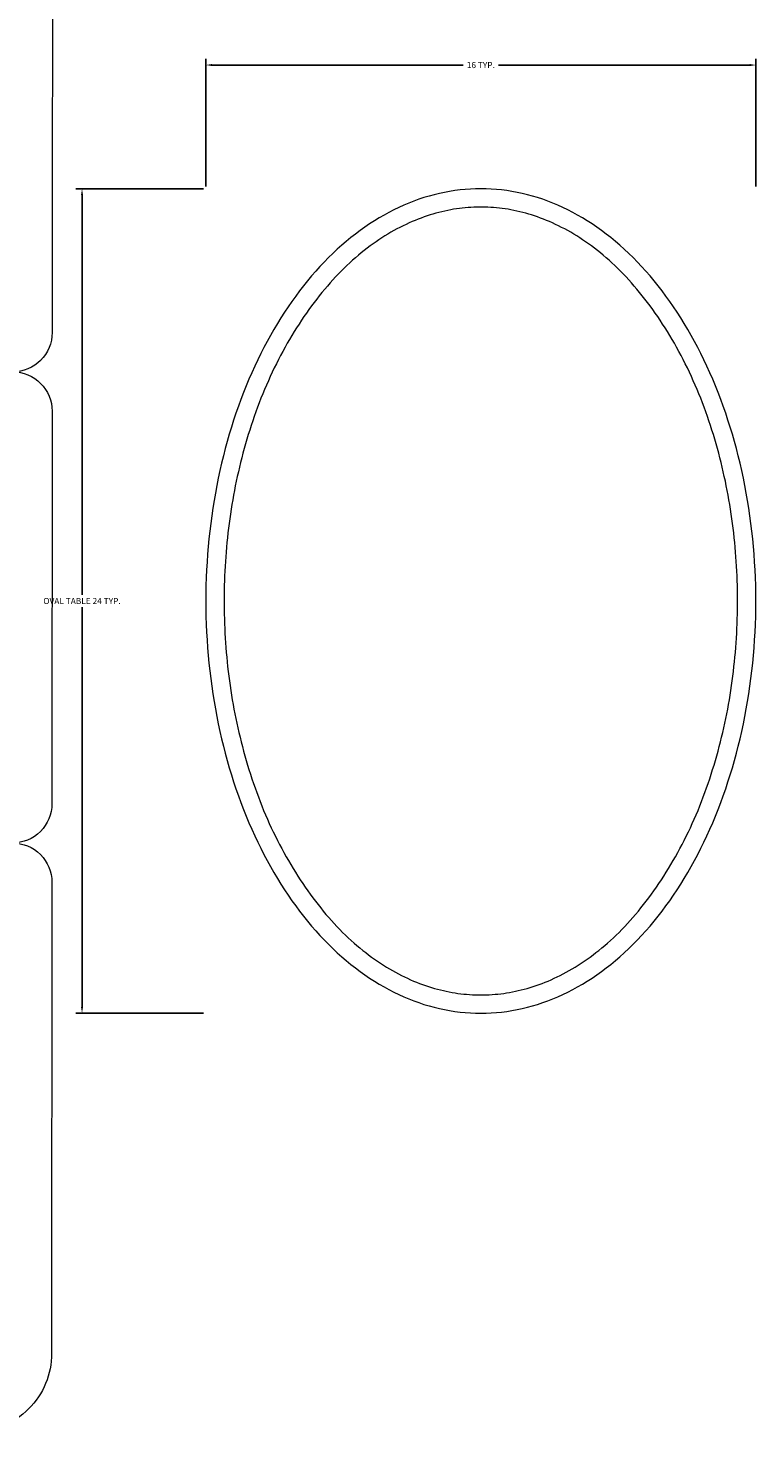
# Model space of a CAD drawing. Units: inches. Extents: x 963 to 2075, y 289 to 2657.
# Tile 84 of 98: x 1533 to 1555, y 2243 to 2284. Entities that reach past the tile are written whole.
import ezdxf

# ---------------------------------------------------------------- set-up
doc = ezdxf.new("R2010")
doc.units = ezdxf.units.IN
doc.layers.add('A-ANNO-DIMS', color=2, linetype='Continuous', lineweight=18)
doc.layers.add('A-FURN', color=8, linetype='Continuous', lineweight=18)
doc.styles.get("Standard").update_dxf_attribs({"font": 'arial.ttf'})
doc.dimstyles.get("Standard").update_dxf_attribs({"dimtxt": 0.18, "dimasz": 0.18, "dimexe": 0.18, "dimexo": 0.0625, "dimgap": 0.09, "dimtad": 0, "dimtih": 1, "dimtoh": 1, "dimdec": 4, "dimzin": 0, "dimdsep": 46, "dimtxsty": 'Standard', "dimcen": 0.09, "dimadec": 0, "dimazin": 0, "dimtfac": 1, "dimtdec": 4, "dimtofl": 0, "dimtmove": 0, "dimatfit": 3, "dimfxl": 1, "dimtolj": 1, "dimtzin": 0, "dimarcsym": 0})

# ---------------------------------------------------------------- blocks, each defined once
blk = doc.blocks.new('SOFA-3SEAT')
at = {"ltscale": 0.03}
blk.add_lwpolyline([(2.442, 16.426, -0.414214), (0.124, 18.743), (0.124, 32.649, -0.414214), (1.283, 33.808, -0.414214), (0.124, 34.967), (0.124, 46.555, -0.414214), (1.283, 47.713, -0.414214), (0.124, 48.872), (0.124, 62.778, -0.414214), (2.442, 65.095), (16.347, 65.095, -0.414214), (18.665, 62.778), (18.665, 18.743, -0.414214), (16.347, 16.426)], format="xyb", close=True, dxfattribs=at)
blk = doc.blocks.new('TABLE-OVAL')
at = {"ltscale": 0.03}
blk.add_polyline3d([(7.656, -0.197, 0), (7.809, -0.194, 0), (7.963, -0.188, 0), (8.116, -0.177, 0), (8.269, -0.162, 0), (8.422, -0.142, 0), (8.575, -0.118, 0), (8.727, -0.09, 0), (8.879, -0.057, 0), (9.031, -0.021, 0), (9.182, 0.021, 0), (9.332, 0.066, 0), (9.482, 0.116, 0), (9.632, 0.17, 0), (9.78, 0.228, 0), (9.928, 0.29, 0), (10.075, 0.357, 0), (10.221, 0.428, 0), (10.366, 0.503, 0), (10.51, 0.582, 0), (10.653, 0.665, 0), (10.796, 0.752, 0), (10.937, 0.843, 0), (11.076, 0.938, 0), (11.215, 1.037, 0), (11.352, 1.14, 0), (11.488, 1.247, 0), (11.623, 1.358, 0), (11.756, 1.472, 0), (11.888, 1.59, 0), (12.018, 1.712, 0), (12.147, 1.838, 0), (12.274, 1.967, 0), (12.399, 2.1, 0), (12.523, 2.237, 0), (12.645, 2.376, 0), (12.765, 2.52, 0), (12.883, 2.666, 0), (13, 2.817, 0), (13.114, 2.97, 0), (13.227, 3.126, 0), (13.337, 3.286, 0), (13.446, 3.449, 0), (13.552, 3.615, 0), (13.657, 3.784, 0), (13.759, 3.955, 0), (13.859, 4.13, 0), (13.957, 4.308, 0), (14.052, 4.488, 0), (14.145, 4.671, 0), (14.236, 4.856, 0), (14.325, 5.044, 0), (14.411, 5.235, 0), (14.495, 5.428, 0), (14.576, 5.623, 0), (14.655, 5.821, 0), (14.731, 6.021, 0), (14.805, 6.222, 0), (14.877, 6.426, 0), (14.945, 6.632, 0), (15.011, 6.84, 0), (15.075, 7.05, 0), (15.135, 7.261, 0), (15.193, 7.475, 0), (15.249, 7.689, 0), (15.301, 7.906, 0), (15.351, 8.123, 0), (15.399, 8.343, 0), (15.443, 8.563, 0), (15.485, 8.785, 0), (15.523, 9.007, 0), (15.559, 9.231, 0), (15.592, 9.456, 0), (15.623, 9.682, 0), (15.65, 9.908, 0), (15.675, 10.136, 0), (15.697, 10.364, 0), (15.715, 10.592, 0), (15.731, 10.821, 0), (15.744, 11.051, 0), (15.755, 11.28, 0), (15.762, 11.51, 0), (15.766, 11.741, 0), (15.768, 11.971, 0), (15.766, 12.201, 0), (15.762, 12.431, 0), (15.755, 12.661, 0), (15.744, 12.891, 0), (15.731, 13.12, 0), (15.715, 13.349, 0), (15.697, 13.578, 0), (15.675, 13.806, 0), (15.65, 14.033, 0), (15.623, 14.26, 0), (15.592, 14.486, 0), (15.559, 14.71, 0), (15.523, 14.934, 0), (15.485, 15.157, 0), (15.443, 15.379, 0), (15.399, 15.599, 0), (15.351, 15.818, 0), (15.301, 16.036, 0), (15.249, 16.252, 0), (15.193, 16.467, 0), (15.135, 16.68, 0), (15.075, 16.892, 0), (15.011, 17.101, 0), (14.945, 17.309, 0), (14.877, 17.515, 0), (14.805, 17.719, 0), (14.731, 17.921, 0), (14.655, 18.121, 0), (14.576, 18.318, 0), (14.495, 18.514, 0), (14.411, 18.707, 0), (14.325, 18.897, 0), (14.236, 19.085, 0), (14.145, 19.271, 0), (14.052, 19.454, 0), (13.957, 19.634, 0), (13.859, 19.811, 0), (13.759, 19.986, 0), (13.657, 20.158, 0), (13.552, 20.327, 0), (13.446, 20.493, 0), (13.337, 20.656, 0), (13.227, 20.815, 0), (13.114, 20.972, 0), (13, 21.125, 0), (12.883, 21.275, 0), (12.765, 21.422, 0), (12.645, 21.565, 0), (12.523, 21.705, 0), (12.399, 21.842, 0), (12.274, 21.974, 0), (12.147, 22.104, 0), (12.018, 22.229, 0), (11.888, 22.351, 0), (11.756, 22.47, 0), (11.623, 22.584, 0), (11.488, 22.695, 0), (11.352, 22.802, 0), (11.215, 22.905, 0), (11.076, 23.004, 0), (10.937, 23.099, 0), (10.796, 23.19, 0), (10.653, 23.277, 0), (10.51, 23.36, 0), (10.366, 23.439, 0), (10.221, 23.514, 0), (10.075, 23.585, 0), (9.928, 23.651, 0), (9.78, 23.714, 0), (9.632, 23.772, 0), (9.482, 23.826, 0), (9.332, 23.876, 0), (9.182, 23.921, 0), (9.031, 23.962, 0), (8.879, 23.999, 0), (8.727, 24.032, 0), (8.575, 24.06, 0), (8.422, 24.084, 0), (8.269, 24.103, 0), (8.116, 24.119, 0), (7.963, 24.13, 0), (7.809, 24.136, 0), (7.656, 24.138, 0), (7.502, 24.136, 0), (7.349, 24.13, 0), (7.196, 24.119, 0), (7.042, 24.103, 0), (6.89, 24.084, 0), (6.737, 24.06, 0), (6.585, 24.032, 0), (6.433, 23.999, 0), (6.281, 23.962, 0), (6.13, 23.921, 0), (5.979, 23.876, 0), (5.83, 23.826, 0), (5.68, 23.772, 0), (5.532, 23.714, 0), (5.384, 23.651, 0), (5.237, 23.585, 0), (5.091, 23.514, 0), (4.946, 23.439, 0), (4.802, 23.36, 0), (4.658, 23.277, 0), (4.516, 23.19, 0), (4.375, 23.099, 0), (4.236, 23.004, 0), (4.097, 22.905, 0), (3.96, 22.802, 0), (3.824, 22.695, 0), (3.689, 22.584, 0), (3.556, 22.47, 0), (3.424, 22.351, 0), (3.294, 22.229, 0), (3.165, 22.104, 0), (3.038, 21.974, 0), (2.913, 21.842, 0), (2.789, 21.705, 0), (2.667, 21.565, 0), (2.547, 21.422, 0), (2.429, 21.275, 0), (2.312, 21.125, 0), (2.198, 20.972, 0), (2.085, 20.815, 0), (1.975, 20.656, 0), (1.866, 20.493, 0), (1.76, 20.327, 0), (1.655, 20.158, 0), (1.553, 19.986, 0), (1.453, 19.811, 0), (1.355, 19.634, 0), (1.26, 19.454, 0), (1.166, 19.271, 0), (1.076, 19.085, 0), (0.987, 18.897, 0), (0.901, 18.707, 0), (0.817, 18.514, 0), (0.736, 18.318, 0), (0.657, 18.121, 0), (0.58, 17.921, 0), (0.507, 17.719, 0), (0.435, 17.515, 0), (0.367, 17.309, 0), (0.301, 17.101, 0), (0.237, 16.892, 0), (0.177, 16.68, 0), (0.118, 16.467, 0), (0.063, 16.252, 0), (0.01, 16.036, 0), (-0.039, 15.818, 0), (-0.087, 15.599, 0), (-0.131, 15.379, 0), (-0.173, 15.157, 0), (-0.211, 14.934, 0), (-0.247, 14.71, 0), (-0.281, 14.486, 0), (-0.311, 14.26, 0), (-0.338, 14.033, 0), (-0.363, 13.806, 0), (-0.385, 13.578, 0), (-0.403, 13.349, 0), (-0.419, 13.12, 0), (-0.432, 12.891, 0), (-0.443, 12.661, 0), (-0.45, 12.431, 0), (-0.454, 12.201, 0), (-0.456, 11.971, 0), (-0.454, 11.741, 0), (-0.45, 11.51, 0), (-0.443, 11.28, 0), (-0.432, 11.051, 0), (-0.419, 10.821, 0), (-0.403, 10.592, 0), (-0.385, 10.364, 0), (-0.363, 10.136, 0), (-0.338, 9.908, 0), (-0.311, 9.682, 0), (-0.281, 9.456, 0), (-0.247, 9.231, 0), (-0.211, 9.007, 0), (-0.173, 8.785, 0), (-0.131, 8.563, 0), (-0.087, 8.343, 0), (-0.039, 8.123, 0), (0.01, 7.906, 0), (0.063, 7.689, 0), (0.118, 7.475, 0), (0.177, 7.261, 0), (0.237, 7.05, 0), (0.301, 6.84, 0), (0.367, 6.632, 0), (0.435, 6.426, 0), (0.507, 6.222, 0), (0.58, 6.021, 0), (0.657, 5.821, 0), (0.736, 5.623, 0), (0.817, 5.428, 0), (0.901, 5.235, 0), (0.987, 5.044, 0), (1.076, 4.856, 0), (1.166, 4.671, 0), (1.26, 4.488, 0), (1.355, 4.308, 0), (1.453, 4.13, 0), (1.553, 3.955, 0), (1.655, 3.784, 0), (1.76, 3.615, 0), (1.866, 3.449, 0), (1.975, 3.286, 0), (2.085, 3.126, 0), (2.198, 2.97, 0), (2.312, 2.817, 0), (2.429, 2.666, 0), (2.547, 2.52, 0), (2.667, 2.376, 0), (2.789, 2.237, 0), (2.913, 2.1, 0), (3.038, 1.967, 0), (3.165, 1.838, 0), (3.294, 1.712, 0), (3.424, 1.59, 0), (3.556, 1.472, 0), (3.689, 1.358, 0), (3.824, 1.247, 0), (3.96, 1.14, 0), (4.097, 1.037, 0), (4.236, 0.938, 0), (4.375, 0.843, 0), (4.516, 0.752, 0), (4.658, 0.665, 0), (4.802, 0.582, 0), (4.946, 0.503, 0), (5.091, 0.428, 0), (5.237, 0.357, 0), (5.384, 0.29, 0), (5.532, 0.228, 0), (5.68, 0.17, 0), (5.83, 0.116, 0), (5.979, 0.066, 0), (6.13, 0.021, 0), (6.281, -0.021, 0), (6.433, -0.057, 0), (6.585, -0.09, 0), (6.737, -0.118, 0), (6.89, -0.142, 0), (7.042, -0.162, 0), (7.196, -0.177, 0), (7.349, -0.188, 0), (7.502, -0.194, 0), (7.656, -0.197, 0)], dxfattribs=at)
blk.add_polyline3d([(7.656, 0.344, 0), (7.739, 0.345, 0), (7.822, 0.347, 0), (7.906, 0.351, 0), (7.99, 0.356, 0), (8.074, 0.362, 0), (8.159, 0.37, 0), (8.244, 0.38, 0), (8.33, 0.391, 0), (8.415, 0.404, 0), (8.501, 0.418, 0), (8.588, 0.434, 0), (8.674, 0.451, 0), (8.761, 0.47, 0), (8.848, 0.491, 0), (8.935, 0.513, 0), (9.023, 0.538, 0), (9.11, 0.563, 0), (9.198, 0.591, 0), (9.286, 0.62, 0), (9.375, 0.651, 0), (9.463, 0.684, 0), (9.552, 0.719, 0), (9.64, 0.755, 0), (9.729, 0.794, 0), (9.818, 0.834, 0), (9.907, 0.876, 0), (9.995, 0.92, 0), (10.084, 0.966, 0), (10.173, 1.013, 0), (10.262, 1.063, 0), (10.35, 1.114, 0), (10.439, 1.167, 0), (10.527, 1.222, 0), (10.615, 1.279, 0), (10.703, 1.338, 0), (10.791, 1.398, 0), (10.878, 1.461, 0), (10.965, 1.525, 0), (11.052, 1.592, 0), (11.139, 1.66, 0), (11.225, 1.73, 0), (11.311, 1.802, 0), (11.396, 1.876, 0), (11.481, 1.952, 0), (11.565, 2.03, 0), (11.649, 2.109, 0), (11.733, 2.191, 0), (11.815, 2.275, 0), (11.898, 2.361, 0), (11.98, 2.448, 0), (12.061, 2.537, 0), (12.141, 2.629, 0), (12.221, 2.721, 0), (12.301, 2.816, 0), (12.379, 2.912, 0), (12.457, 3.01, 0), (12.535, 3.11, 0), (12.611, 3.211, 0), (12.687, 3.314, 0), (12.762, 3.418, 0), (12.836, 3.524, 0), (12.909, 3.632, 0), (12.982, 3.741, 0), (13.053, 3.851, 0), (13.124, 3.963, 0), (13.194, 4.076, 0), (13.262, 4.191, 0), (13.33, 4.307, 0), (13.397, 4.424, 0), (13.463, 4.543, 0), (13.528, 4.662, 0), (13.591, 4.783, 0), (13.654, 4.906, 0), (13.716, 5.029, 0), (13.776, 5.154, 0), (13.835, 5.279, 0), (13.893, 5.406, 0), (13.95, 5.534, 0), (14.006, 5.663, 0), (14.061, 5.792, 0), (14.114, 5.923, 0), (14.166, 6.055, 0), (14.217, 6.188, 0), (14.266, 6.321, 0), (14.314, 6.455, 0), (14.361, 6.589, 0), (14.406, 6.723, 0), (14.45, 6.858, 0), (14.493, 6.993, 0), (14.535, 7.129, 0), (14.575, 7.265, 0), (14.614, 7.401, 0), (14.652, 7.537, 0), (14.688, 7.674, 0), (14.724, 7.811, 0), (14.758, 7.948, 0), (14.791, 8.086, 0), (14.822, 8.223, 0), (14.852, 8.361, 0), (14.882, 8.5, 0), (14.909, 8.638, 0), (14.936, 8.777, 0), (14.961, 8.916, 0), (14.986, 9.055, 0), (15.009, 9.194, 0), (15.031, 9.334, 0), (15.051, 9.473, 0), (15.071, 9.613, 0), (15.089, 9.753, 0), (15.106, 9.893, 0), (15.122, 10.033, 0), (15.137, 10.174, 0), (15.151, 10.314, 0), (15.163, 10.455, 0), (15.175, 10.596, 0), (15.185, 10.736, 0), (15.194, 10.877, 0), (15.202, 11.018, 0), (15.209, 11.159, 0), (15.215, 11.3, 0), (15.219, 11.441, 0), (15.223, 11.583, 0), (15.225, 11.724, 0), (15.227, 11.865, 0), (15.227, 12.006, 0), (15.226, 12.147, 0), (15.224, 12.288, 0), (15.221, 12.43, 0), (15.217, 12.571, 0), (15.212, 12.712, 0), (15.205, 12.853, 0), (15.198, 12.994, 0), (15.19, 13.135, 0), (15.18, 13.276, 0), (15.169, 13.416, 0), (15.157, 13.557, 0), (15.144, 13.698, 0), (15.13, 13.838, 0), (15.114, 13.978, 0), (15.098, 14.119, 0), (15.08, 14.259, 0), (15.061, 14.399, 0), (15.041, 14.538, 0), (15.02, 14.678, 0), (14.997, 14.817, 0), (14.974, 14.956, 0), (14.949, 15.095, 0), (14.923, 15.234, 0), (14.896, 15.373, 0), (14.867, 15.511, 0), (14.837, 15.649, 0), (14.806, 15.787, 0), (14.774, 15.925, 0), (14.741, 16.062, 0), (14.706, 16.199, 0), (14.67, 16.336, 0), (14.633, 16.473, 0), (14.595, 16.609, 0), (14.555, 16.745, 0), (14.514, 16.881, 0), (14.472, 17.016, 0), (14.428, 17.151, 0), (14.384, 17.286, 0), (14.338, 17.42, 0), (14.29, 17.554, 0), (14.241, 17.687, 0), (14.191, 17.821, 0), (14.14, 17.953, 0), (14.087, 18.084, 0), (14.034, 18.214, 0), (13.978, 18.344, 0), (13.922, 18.472, 0), (13.865, 18.599, 0), (13.806, 18.725, 0), (13.746, 18.85, 0), (13.685, 18.974, 0), (13.623, 19.097, 0), (13.56, 19.219, 0), (13.495, 19.339, 0), (13.43, 19.458, 0), (13.364, 19.576, 0), (13.296, 19.693, 0), (13.228, 19.808, 0), (13.159, 19.922, 0), (13.089, 20.035, 0), (13.017, 20.146, 0), (12.945, 20.255, 0), (12.873, 20.364, 0), (12.799, 20.47, 0), (12.724, 20.576, 0), (12.649, 20.679, 0), (12.573, 20.781, 0), (12.496, 20.882, 0), (12.418, 20.981, 0), (12.34, 21.078, 0), (12.261, 21.173, 0), (12.182, 21.267, 0), (12.101, 21.359, 0), (12.02, 21.449, 0), (11.939, 21.537, 0), (11.857, 21.624, 0), (11.774, 21.709, 0), (11.691, 21.791, 0), (11.607, 21.872, 0), (11.523, 21.951, 0), (11.438, 22.028, 0), (11.353, 22.103, 0), (11.268, 22.176, 0), (11.182, 22.247, 0), (11.095, 22.316, 0), (11.009, 22.383, 0), (10.922, 22.449, 0), (10.835, 22.512, 0), (10.747, 22.574, 0), (10.659, 22.633, 0), (10.571, 22.691, 0), (10.483, 22.747, 0), (10.395, 22.801, 0), (10.306, 22.854, 0), (10.217, 22.904, 0), (10.129, 22.952, 0), (10.04, 22.999, 0), (9.951, 23.044, 0), (9.862, 23.087, 0), (9.773, 23.128, 0), (9.685, 23.167, 0), (9.596, 23.205, 0), (9.507, 23.24, 0), (9.419, 23.274, 0), (9.331, 23.306, 0), (9.242, 23.336, 0), (9.154, 23.365, 0), (9.067, 23.391, 0), (8.979, 23.416, 0), (8.892, 23.44, 0), (8.804, 23.461, 0), (8.718, 23.481, 0), (8.631, 23.499, 0), (8.544, 23.516, 0), (8.458, 23.531, 0), (8.373, 23.545, 0), (8.287, 23.557, 0), (8.202, 23.567, 0), (8.117, 23.576, 0), (8.032, 23.583, 0), (7.948, 23.589, 0), (7.864, 23.593, 0), (7.781, 23.596, 0), (7.697, 23.597, 0), (7.615, 23.597, 0), (7.531, 23.596, 0), (7.448, 23.593, 0), (7.364, 23.589, 0), (7.28, 23.583, 0), (7.195, 23.576, 0), (7.11, 23.567, 0), (7.025, 23.557, 0), (6.939, 23.545, 0), (6.854, 23.531, 0), (6.767, 23.516, 0), (6.681, 23.499, 0), (6.594, 23.481, 0), (6.507, 23.461, 0), (6.42, 23.44, 0), (6.333, 23.416, 0), (6.245, 23.391, 0), (6.158, 23.365, 0), (6.07, 23.336, 0), (5.981, 23.306, 0), (5.893, 23.274, 0), (5.805, 23.24, 0), (5.716, 23.205, 0), (5.627, 23.167, 0), (5.539, 23.128, 0), (5.45, 23.087, 0), (5.361, 23.044, 0), (5.272, 22.999, 0), (5.183, 22.952, 0), (5.095, 22.904, 0), (5.006, 22.854, 0), (4.917, 22.801, 0), (4.829, 22.747, 0), (4.741, 22.691, 0), (4.653, 22.633, 0), (4.565, 22.574, 0), (4.477, 22.512, 0), (4.39, 22.449, 0), (4.303, 22.383, 0), (4.216, 22.316, 0), (4.13, 22.247, 0), (4.044, 22.176, 0), (3.959, 22.103, 0), (3.874, 22.028, 0), (3.789, 21.951, 0), (3.705, 21.872, 0), (3.621, 21.791, 0), (3.538, 21.709, 0), (3.455, 21.624, 0), (3.373, 21.537, 0), (3.292, 21.449, 0), (3.211, 21.359, 0), (3.13, 21.267, 0), (3.051, 21.173, 0), (2.972, 21.078, 0), (2.893, 20.981, 0), (2.816, 20.882, 0), (2.739, 20.781, 0), (2.663, 20.679, 0), (2.588, 20.576, 0), (2.513, 20.47, 0), (2.439, 20.364, 0), (2.366, 20.255, 0), (2.294, 20.146, 0), (2.223, 20.035, 0), (2.153, 19.922, 0), (2.084, 19.808, 0), (2.016, 19.693, 0), (1.948, 19.576, 0), (1.882, 19.458, 0), (1.817, 19.339, 0), (1.752, 19.219, 0), (1.689, 19.097, 0), (1.627, 18.974, 0), (1.566, 18.85, 0), (1.506, 18.725, 0), (1.447, 18.599, 0), (1.39, 18.472, 0), (1.334, 18.344, 0), (1.278, 18.214, 0), (1.225, 18.084, 0), (1.172, 17.953, 0), (1.121, 17.821, 0), (1.071, 17.687, 0), (1.022, 17.554, 0), (0.974, 17.42, 0), (0.928, 17.286, 0), (0.884, 17.151, 0), (0.84, 17.016, 0), (0.798, 16.881, 0), (0.757, 16.745, 0), (0.717, 16.609, 0), (0.679, 16.473, 0), (0.642, 16.336, 0), (0.606, 16.199, 0), (0.571, 16.062, 0), (0.538, 15.925, 0), (0.505, 15.787, 0), (0.475, 15.649, 0), (0.445, 15.511, 0), (0.416, 15.373, 0), (0.389, 15.234, 0), (0.363, 15.095, 0), (0.338, 14.956, 0), (0.315, 14.817, 0), (0.292, 14.678, 0), (0.271, 14.538, 0), (0.251, 14.399, 0), (0.232, 14.259, 0), (0.214, 14.119, 0), (0.198, 13.978, 0), (0.182, 13.838, 0), (0.168, 13.698, 0), (0.155, 13.557, 0), (0.143, 13.416, 0), (0.132, 13.276, 0), (0.122, 13.135, 0), (0.114, 12.994, 0), (0.106, 12.853, 0), (0.1, 12.712, 0), (0.095, 12.571, 0), (0.091, 12.43, 0), (0.088, 12.288, 0), (0.086, 12.147, 0), (0.085, 12.006, 0), (0.085, 11.865, 0), (0.087, 11.724, 0), (0.089, 11.583, 0), (0.093, 11.441, 0), (0.097, 11.3, 0), (0.103, 11.159, 0), (0.11, 11.018, 0), (0.118, 10.877, 0), (0.127, 10.736, 0), (0.137, 10.596, 0), (0.149, 10.455, 0), (0.161, 10.314, 0), (0.175, 10.174, 0), (0.19, 10.033, 0), (0.206, 9.893, 0), (0.223, 9.753, 0), (0.241, 9.613, 0), (0.261, 9.473, 0), (0.281, 9.334, 0), (0.303, 9.194, 0), (0.326, 9.055, 0), (0.35, 8.916, 0), (0.376, 8.777, 0), (0.403, 8.638, 0), (0.43, 8.5, 0), (0.46, 8.361, 0), (0.49, 8.223, 0), (0.521, 8.086, 0), (0.554, 7.948, 0), (0.588, 7.811, 0), (0.623, 7.674, 0), (0.66, 7.537, 0), (0.698, 7.401, 0), (0.737, 7.265, 0), (0.777, 7.129, 0), (0.819, 6.993, 0), (0.862, 6.858, 0), (0.906, 6.723, 0), (0.951, 6.589, 0), (0.998, 6.455, 0), (1.046, 6.321, 0), (1.095, 6.188, 0), (1.146, 6.055, 0), (1.198, 5.923, 0), (1.251, 5.792, 0), (1.306, 5.663, 0), (1.362, 5.534, 0), (1.418, 5.406, 0), (1.477, 5.279, 0), (1.536, 5.154, 0), (1.596, 5.029, 0), (1.658, 4.906, 0), (1.721, 4.783, 0), (1.784, 4.662, 0), (1.849, 4.543, 0), (1.915, 4.424, 0), (1.982, 4.307, 0), (2.05, 4.191, 0), (2.118, 4.076, 0), (2.188, 3.963, 0), (2.259, 3.851, 0), (2.33, 3.741, 0), (2.403, 3.632, 0), (2.476, 3.524, 0), (2.55, 3.418, 0), (2.625, 3.314, 0), (2.701, 3.211, 0), (2.777, 3.11, 0), (2.855, 3.01, 0), (2.933, 2.912, 0), (3.011, 2.816, 0), (3.09, 2.721, 0), (3.17, 2.629, 0), (3.251, 2.537, 0), (3.332, 2.448, 0), (3.414, 2.361, 0), (3.497, 2.275, 0), (3.579, 2.191, 0), (3.663, 2.109, 0), (3.747, 2.03, 0), (3.831, 1.952, 0), (3.916, 1.876, 0), (4.001, 1.802, 0), (4.087, 1.73, 0), (4.173, 1.66, 0), (4.26, 1.592, 0), (4.347, 1.525, 0), (4.434, 1.461, 0), (4.521, 1.398, 0), (4.609, 1.338, 0), (4.697, 1.279, 0), (4.785, 1.222, 0), (4.873, 1.167, 0), (4.962, 1.114, 0), (5.05, 1.063, 0), (5.139, 1.013, 0), (5.228, 0.966, 0), (5.316, 0.92, 0), (5.405, 0.876, 0), (5.494, 0.834, 0), (5.583, 0.794, 0), (5.672, 0.755, 0), (5.76, 0.719, 0), (5.849, 0.684, 0), (5.937, 0.651, 0), (6.026, 0.62, 0), (6.114, 0.591, 0), (6.201, 0.563, 0), (6.289, 0.538, 0), (6.377, 0.513, 0), (6.464, 0.491, 0), (6.551, 0.47, 0), (6.638, 0.451, 0), (6.724, 0.434, 0), (6.811, 0.418, 0), (6.897, 0.404, 0), (6.982, 0.391, 0), (7.068, 0.38, 0), (7.153, 0.37, 0), (7.237, 0.362, 0), (7.322, 0.356, 0), (7.406, 0.351, 0), (7.49, 0.347, 0), (7.573, 0.345, 0), (7.656, 0.344, 0)])
blk = doc.blocks.new('*D18')
at = {"layer": 'A-ANNO-DIMS', "color": 0, "lineweight": -2, "transparency": 16777216}
for p, q in [((1538.337, 2279.539), (1534.57, 2279.539)), ((1534.75, 2279.359), (1534.75, 2267.555)), ((1534.75, 2255.385), (1534.75, 2267.189)), ((1538.337, 2255.205), (1534.57, 2255.205))]:
    blk.add_line(p, q, dxfattribs=at)
at = {"layer": 'A-ANNO-DIMS', "color": 0, "transparency": 16777216}
for points in [[(1534.72, 2279.359), (1534.78, 2279.359), (1534.75, 2279.539)], [(1534.72, 2255.385), (1534.78, 2255.385), (1534.75, 2255.205)]]:
    blk.add_solid(points, dxfattribs=at)
at = {"layer": 'Defpoints', "color": 0, "transparency": 16777216}
for p in [(1534.75, 2279.539), (1538.4, 2279.539), (1538.4, 2255.205)]:
    blk.add_point(p, dxfattribs=at)
at = {"layer": 'A-ANNO-DIMS', "color": 0, "transparency": 16777216, "insert": (1534.75, 2267.372), "char_height": 0.18, "attachment_point": 5}
blk.add_mtext('\\A1;OVAL TABLE 24 TYP.', dxfattribs=at)
blk = doc.blocks.new('*D19')
at = {"layer": 'A-ANNO-DIMS', "color": 0, "lineweight": -2, "transparency": 16777216}
for p, q in [((1538.4, 2279.602), (1538.4, 2283.37)), ((1538.58, 2283.19), (1545.992, 2283.19)), ((1554.443, 2283.19), (1547.031, 2283.19)), ((1554.623, 2279.602), (1554.623, 2283.37))]:
    blk.add_line(p, q, dxfattribs=at)
at = {"layer": 'A-ANNO-DIMS', "color": 0, "transparency": 16777216}
for points in [[(1538.58, 2283.22), (1538.58, 2283.16), (1538.4, 2283.19)], [(1554.443, 2283.22), (1554.443, 2283.16), (1554.623, 2283.19)]]:
    blk.add_solid(points, dxfattribs=at)
at = {"layer": 'Defpoints', "color": 0, "transparency": 16777216}
for p in [(1554.623, 2283.19), (1538.4, 2279.539), (1554.623, 2279.539)]:
    blk.add_point(p, dxfattribs=at)
at = {"layer": 'A-ANNO-DIMS', "color": 0, "transparency": 16777216, "insert": (1546.511, 2283.19), "char_height": 0.18, "attachment_point": 5}
blk.add_mtext('\\A1;16 TYP.', dxfattribs=at)

msp = doc.modelspace()

# ---------------------------------------------------------------- block references
at = {"layer": 'A-FURN', "rotation": 179.9690487318625}
msp.add_blockref('SOFA-3SEAT', (1534.012, 2307.942), dxfattribs=at)
at = {"layer": 'A-FURN'}
msp.add_blockref('TABLE-OVAL', (1538.855, 2255.401), dxfattribs=at)

# ---------------------------------------------------------------- dimensions: what is measured, and where the dimension line sits
at = {"layer": 'A-ANNO-DIMS'}
dim = msp.add_linear_dim(base=(1554.623, 2283.19), p1=(1538.4, 2279.539), p2=(1554.623, 2279.539), text='<> TYP.', dimstyle='Standard', override={"dimdec": 0, "dimlfac": 1, "dimrnd": 0, "dimzin": 0, "dimdsep": 46, "dimlunit": 2}, dxfattribs=at)
dim.commit()
dim.dimension.update_dxf_attribs({"geometry": '*D19', "text_midpoint": (1546.511, 2283.19)})
dim = msp.add_linear_dim(base=(1534.75, 2279.539), p1=(1538.4, 2255.205), p2=(1538.4, 2279.539), angle=90, text='OVAL TABLE <> TYP.', dimstyle='Standard', override={"dimdec": 0, "dimlfac": 1, "dimrnd": 0, "dimzin": 0, "dimdsep": 46, "dimlunit": 2}, dxfattribs=at)
dim.commit()
dim.dimension.update_dxf_attribs({"geometry": '*D18', "text_midpoint": (1534.75, 2267.372)})

doc.saveas('drawing.dxf')
